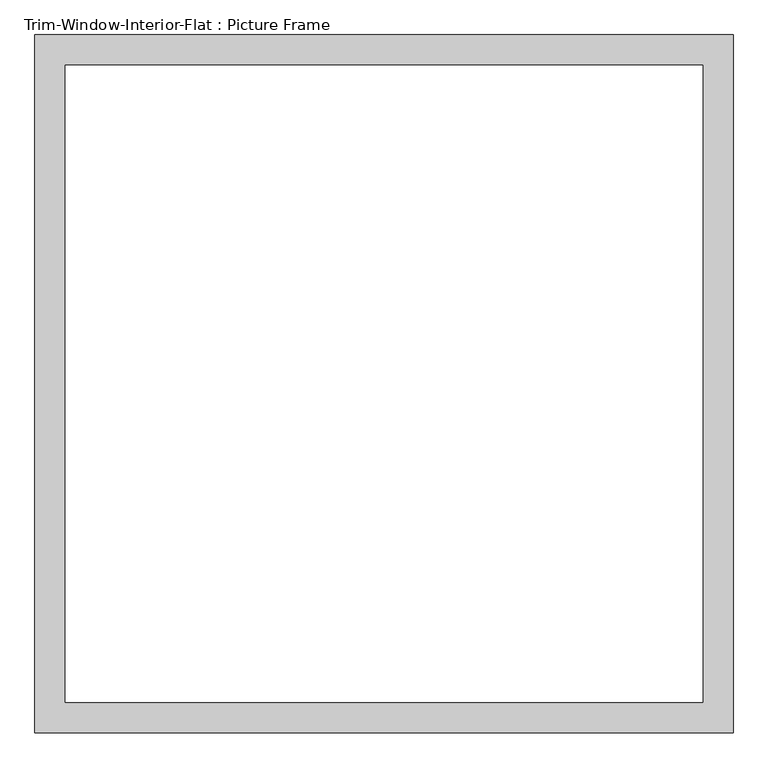
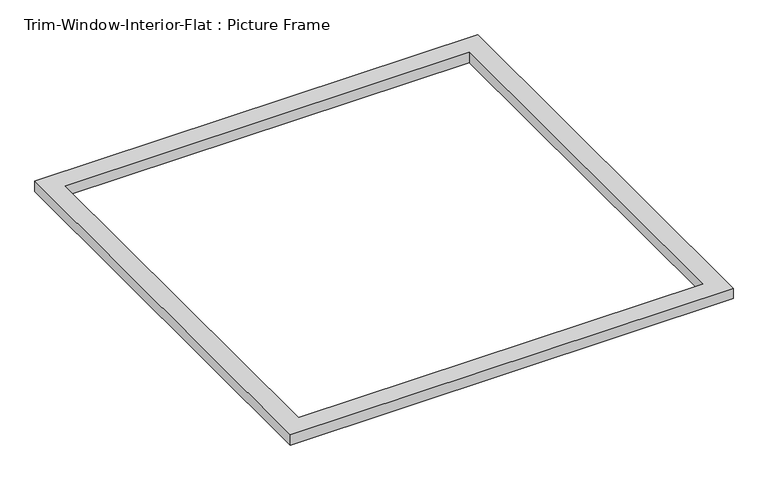
"""IFC4 building model written with IfcOpenShell, lengths in millimetres: proxy geometry, Trim-Window-Interior-Flat : Picture Frame."""

from ifc_helpers import new_model, si_unit, origin, origin_with_axes, place, context, project, spatial, polyline, outline, extrude, source, transform, mapped, element, save


def trim_window_interior_flat_picture_frame_f1e0b15b(model_context):
    return source(origin(), model_context, "Body", "SweptSolid", [
        extrude(outline(polyline([(654.05, 44.45), (654.05, -1263.65), (-654.05, -1263.65), (-654.05, 44.45), (654.05, 44.45)]), holes=[polyline([(596.9, -12.7), (-596.9, -12.7), (-596.9, -1206.5), (596.9, -1206.5), (596.9, -12.7)])]), origin_with_axes(), (0.0, 0.0, 1.0), 31.75),
    ])


if __name__ == "__main__":
    model = new_model("IFC4")
    model_context = context("Model", 3, world=origin())
    ifc_project = project(units=[si_unit("LENGTHUNIT", "METRE", prefix="MILLI")], contexts=[model_context])
    site = spatial("IfcSite", under=ifc_project)
    building = spatial("IfcBuilding", under=site)
    placement = place(None, origin())
    trim_window_interior_flat_picture_frame_shape = trim_window_interior_flat_picture_frame_f1e0b15b(model_context)
    element("IfcBuildingElementProxy", 1, Name="Trim-Window-Interior-Flat : Picture Frame", ObjectType="Trim-Window-Interior-Flat : Picture Frame", at=placement, inside=building, context=model_context, shape_type="MappedRepresentation", body=[
        mapped(trim_window_interior_flat_picture_frame_shape, transform((0.0, 0.0, 0.0), x_axis=(1.0, 0.0, 0.0), y_axis=(0.0, 1.0, 0.0), z_axis=(0.0, 0.0, 1.0))),
    ])
    save(model, "model.ifc")

# Revit data of these elements
# Type "Trim-Window-Interior-Flat : Picture Frame"
#   Trim Thickness_Picture Frame = 0' - 1 1/4"
#   Trim Width = 0' - 2 1/4"
#   Trim Thickness_with Sill = 0' - 0 3/4"
#   Sill Thickness = 0' - 1 1/4"
#   Opening Width [instance default] = 2' - 0"
#   Opening Height [instance default] = 3' - 0"
#   Default Elevation = 4' - 0"
#   Sill = no
#   Picture Frame = yes
#   Trim Material [instance default] = none
# Element 1 (IfcBuildingElementProxy, "Trim-Window-Interior-Flat : Picture Frame")
#   Opening Width = 4' - 0"
#   Opening Height = 4' - 0"
#   Trim Material = Wood - Stained
#   Materials on its faces: "Wood - Stained"
# Materials
#   "Wood - Stained": class "Wood", colour RGB 224 178 126, transparency 0, Cost = 0
